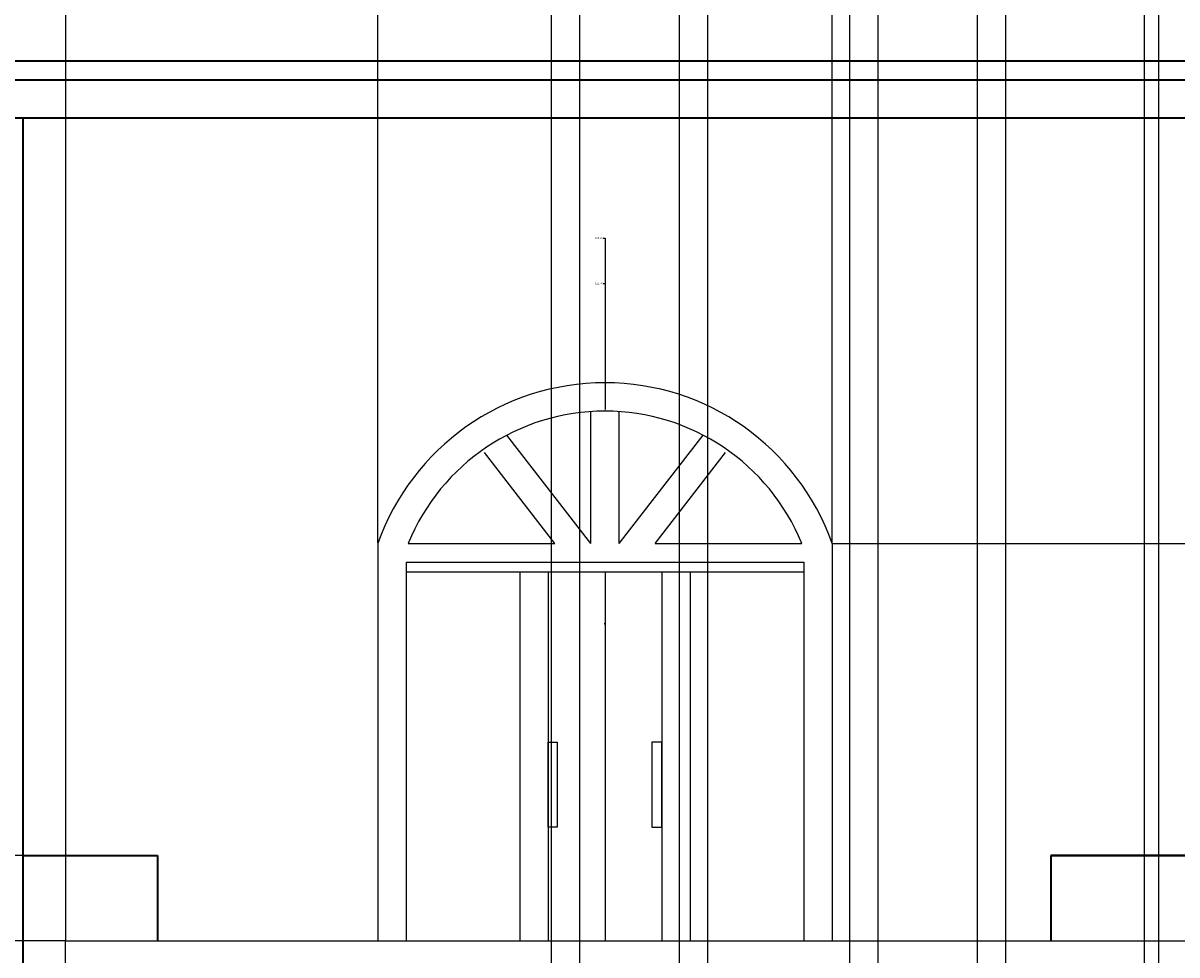
# Model space of a CAD drawing. Units: inches. Extents: x 2612 to 2948, y 481 to 865.
# Tile 3 of 7: x 2708 to 2830, y 561 to 659. Entities that reach past the tile are written whole.
import ezdxf

# ---------------------------------------------------------------- set-up
doc = ezdxf.new("R2010")
doc.units = ezdxf.units.IN
for name, color, linetype, lineweight in [('A-ANNO-DIMS', 2, 'Continuous', 18), ('A-DOOR', 4, 'Continuous', 25), ('A-ELEV', 7, 'Continuous', 35)]:
    doc.layers.add(name, color=color, linetype=linetype, lineweight=lineweight)
doc.styles.get("Standard").update_dxf_attribs({"font": 'arial.ttf'})
doc.dimstyles.get("Standard").update_dxf_attribs({"dimtxt": 0.18, "dimasz": 0.18, "dimexe": 0.18, "dimexo": 0.0625, "dimgap": 0.09, "dimtad": 0, "dimtih": 1, "dimtoh": 1, "dimdec": 4, "dimzin": 0, "dimdsep": 46, "dimtxsty": 'Standard', "dimcen": 0.09, "dimadec": 0, "dimazin": 0, "dimtfac": 1, "dimtdec": 4, "dimtofl": 0, "dimtmove": 0, "dimatfit": 3, "dimfxl": 1, "dimtolj": 1, "dimtzin": 0, "dimarcsym": 0})

# ---------------------------------------------------------------- blocks, each defined once
blk = doc.blocks.new('*D22')
at = {"layer": 'A-ANNO-DIMS', "color": 0, "lineweight": -2, "transparency": 16777216}
for p, q in [((2708.31, 648.98), (2708.31, 481.26)), ((2831.31, 570.98), (2831.31, 481.26)), ((2708.49, 481.44), (2769.53, 481.44)), ((2831.13, 481.44), (2770.09, 481.44))]:
    blk.add_line(p, q, dxfattribs=at)
at = {"layer": 'A-ANNO-DIMS', "color": 0, "transparency": 16777216}
for points in [[(2708.49, 481.47), (2708.49, 481.41), (2708.31, 481.44)], [(2831.13, 481.47), (2831.13, 481.41), (2831.31, 481.44)]]:
    blk.add_solid(points, dxfattribs=at)
at = {"layer": 'Defpoints', "color": 0, "transparency": 16777216}
for p in [(2708.31, 649.04), (2831.31, 571.04), (2831.31, 481.44)]:
    blk.add_point(p, dxfattribs=at)
at = {"layer": 'A-ANNO-DIMS', "color": 0, "transparency": 16777216, "insert": (2769.81, 481.44), "char_height": 0.18, "attachment_point": 5}
blk.add_mtext('\\A1;123', dxfattribs=at)
blk = doc.blocks.new('*D49')
at = {"layer": 'A-ANNO-DIMS', "color": 0, "lineweight": -2, "transparency": 16777216}
for p, q in [((2712.81, 562.11), (2712.81, 864.82)), ((2712.99, 864.64), (2729.09, 864.64)), ((2745.63, 864.64), (2729.53, 864.64)), ((2745.81, 604.11), (2745.81, 864.82))]:
    blk.add_line(p, q, dxfattribs=at)
at = {"layer": 'A-ANNO-DIMS', "color": 0, "transparency": 16777216}
for points in [[(2712.99, 864.67), (2712.99, 864.61), (2712.81, 864.64)], [(2745.63, 864.67), (2745.63, 864.61), (2745.81, 864.64)]]:
    blk.add_solid(points, dxfattribs=at)
at = {"layer": 'Defpoints', "color": 0, "transparency": 16777216}
for p in [(2745.81, 864.64), (2745.81, 604.04), (2712.81, 562.04)]:
    blk.add_point(p, dxfattribs=at)
at = {"layer": 'A-ANNO-DIMS', "color": 0, "transparency": 16777216, "insert": (2729.31, 864.64), "char_height": 0.18, "attachment_point": 5}
blk.add_mtext('\\A1;33', dxfattribs=at)
blk = doc.blocks.new('*D50')
at = {"layer": 'A-ANNO-DIMS', "color": 0, "lineweight": -2, "transparency": 16777216}
for p, q in [((2745.81, 604.11), (2745.81, 864.82)), ((2745.99, 864.64), (2769.58, 864.64)), ((2793.63, 864.64), (2770.03, 864.64)), ((2793.81, 604.11), (2793.81, 864.82))]:
    blk.add_line(p, q, dxfattribs=at)
at = {"layer": 'A-ANNO-DIMS', "color": 0, "transparency": 16777216}
for points in [[(2745.99, 864.67), (2745.99, 864.61), (2745.81, 864.64)], [(2793.63, 864.67), (2793.63, 864.61), (2793.81, 864.64)]]:
    blk.add_solid(points, dxfattribs=at)
at = {"layer": 'Defpoints', "color": 0, "transparency": 16777216}
for p in [(2793.81, 864.64), (2745.81, 604.04), (2793.81, 604.04)]:
    blk.add_point(p, dxfattribs=at)
at = {"layer": 'A-ANNO-DIMS', "color": 0, "transparency": 16777216, "insert": (2769.81, 864.64), "char_height": 0.18, "attachment_point": 5}
blk.add_mtext('\\A1;48', dxfattribs=at)
blk = doc.blocks.new('*D51')
at = {"layer": 'A-ANNO-DIMS', "color": 0, "lineweight": -2, "transparency": 16777216}
for p, q in [((2793.81, 604.11), (2793.81, 864.82)), ((2793.99, 864.64), (2810.09, 864.64)), ((2826.63, 864.64), (2810.53, 864.64)), ((2826.81, 562.11), (2826.81, 864.82))]:
    blk.add_line(p, q, dxfattribs=at)
at = {"layer": 'A-ANNO-DIMS', "color": 0, "transparency": 16777216}
for points in [[(2793.99, 864.67), (2793.99, 864.61), (2793.81, 864.64)], [(2826.63, 864.67), (2826.63, 864.61), (2826.81, 864.64)]]:
    blk.add_solid(points, dxfattribs=at)
at = {"layer": 'Defpoints', "color": 0, "transparency": 16777216}
for p in [(2826.81, 864.64), (2793.81, 604.04), (2826.81, 562.04)]:
    blk.add_point(p, dxfattribs=at)
at = {"layer": 'A-ANNO-DIMS', "color": 0, "transparency": 16777216, "insert": (2810.31, 864.64), "char_height": 0.18, "attachment_point": 5}
blk.add_mtext('\\A1;33', dxfattribs=at)
blk = doc.blocks.new('*D62')
at = {"layer": 'A-ANNO-DIMS', "color": 0, "lineweight": -2, "transparency": 16777216}
for p, q in [((2712.74, 562.04), (2612.53, 562.04)), ((2612.71, 561.86), (2612.71, 560.73)), ((2612.71, 559.22), (2612.71, 560.36)), ((2715.74, 559.04), (2612.53, 559.04))]:
    blk.add_line(p, q, dxfattribs=at)
at = {"layer": 'A-ANNO-DIMS', "color": 0, "transparency": 16777216}
for points in [[(2612.68, 561.86), (2612.74, 561.86), (2612.71, 562.04)], [(2612.68, 559.22), (2612.74, 559.22), (2612.71, 559.04)]]:
    blk.add_solid(points, dxfattribs=at)
at = {"layer": 'Defpoints', "color": 0, "transparency": 16777216}
for p in [(2612.71, 562.04), (2712.81, 562.04), (2715.81, 559.04)]:
    blk.add_point(p, dxfattribs=at)
at = {"layer": 'A-ANNO-DIMS', "color": 0, "transparency": 16777216, "insert": (2612.71, 560.54), "char_height": 0.18, "attachment_point": 5}
blk.add_mtext('\\A1;3', dxfattribs=at)
blk = doc.blocks.new('*D63')
at = {"layer": 'A-ANNO-DIMS', "color": 0, "lineweight": -2, "transparency": 16777216}
for p, q in [((2722.45, 571.04), (2612.53, 571.04)), ((2612.71, 570.86), (2612.71, 566.73)), ((2612.71, 562.22), (2612.71, 566.36)), ((2712.74, 562.04), (2612.53, 562.04))]:
    blk.add_line(p, q, dxfattribs=at)
at = {"layer": 'A-ANNO-DIMS', "color": 0, "transparency": 16777216}
for points in [[(2612.68, 570.86), (2612.74, 570.86), (2612.71, 571.04)], [(2612.68, 562.22), (2612.74, 562.22), (2612.71, 562.04)]]:
    blk.add_solid(points, dxfattribs=at)
at = {"layer": 'Defpoints', "color": 0, "transparency": 16777216}
for p in [(2612.71, 571.04), (2722.51, 571.04), (2712.81, 562.04)]:
    blk.add_point(p, dxfattribs=at)
at = {"layer": 'A-ANNO-DIMS', "color": 0, "transparency": 16777216, "insert": (2612.71, 566.54), "char_height": 0.18, "attachment_point": 5}
blk.add_mtext('\\A1;9', dxfattribs=at)
blk = doc.blocks.new('*D64')
at = {"layer": 'A-ANNO-DIMS', "color": 0, "lineweight": -2, "transparency": 16777216}
for p, q in [((2826.87, 562.04), (2948.09, 562.04)), ((2947.91, 561.86), (2947.91, 530.73)), ((2947.91, 499.22), (2947.91, 530.36)), ((2826.87, 499.04), (2948.09, 499.04))]:
    blk.add_line(p, q, dxfattribs=at)
at = {"layer": 'A-ANNO-DIMS', "color": 0, "transparency": 16777216}
for points in [[(2947.88, 561.86), (2947.94, 561.86), (2947.91, 562.04)], [(2947.88, 499.22), (2947.94, 499.22), (2947.91, 499.04)]]:
    blk.add_solid(points, dxfattribs=at)
at = {"layer": 'Defpoints', "color": 0, "transparency": 16777216}
for p in [(2826.81, 562.04), (2947.91, 562.04), (2826.81, 499.04)]:
    blk.add_point(p, dxfattribs=at)
at = {"layer": 'A-ANNO-DIMS', "color": 0, "transparency": 16777216, "insert": (2947.91, 530.54), "char_height": 0.18, "attachment_point": 5}
blk.add_mtext('\\A1;63', dxfattribs=at)
blk = doc.blocks.new('*D65')
at = {"layer": 'A-ANNO-DIMS', "color": 0, "lineweight": -2, "transparency": 16777216}
for p, q in [((2793.87, 604.04), (2948.09, 604.04)), ((2947.91, 603.86), (2947.91, 583.22)), ((2947.91, 562.22), (2947.91, 582.86)), ((2793.87, 562.04), (2948.09, 562.04))]:
    blk.add_line(p, q, dxfattribs=at)
at = {"layer": 'A-ANNO-DIMS', "color": 0, "transparency": 16777216}
for points in [[(2947.88, 603.86), (2947.94, 603.86), (2947.91, 604.04)], [(2947.88, 562.22), (2947.94, 562.22), (2947.91, 562.04)]]:
    blk.add_solid(points, dxfattribs=at)
at = {"layer": 'Defpoints', "color": 0, "transparency": 16777216}
for p in [(2793.81, 604.04), (2947.91, 604.04), (2793.81, 562.04)]:
    blk.add_point(p, dxfattribs=at)
at = {"layer": 'A-ANNO-DIMS', "color": 0, "transparency": 16777216, "insert": (2947.91, 583.04), "char_height": 0.18, "attachment_point": 5}
blk.add_mtext('\\A1;42', dxfattribs=at)
blk = doc.blocks.new('*D66')
at = {"layer": 'A-ANNO-DIMS', "color": 0, "lineweight": -2, "transparency": 16777216}
for p, q in [((2767.13, 711.98), (2767.13, 481.26)), ((2764.13, 708.98), (2764.13, 481.26)), ((2764.31, 481.44), (2765.48, 481.44)), ((2766.95, 481.44), (2765.78, 481.44))]:
    blk.add_line(p, q, dxfattribs=at)
at = {"layer": 'A-ANNO-DIMS', "color": 0, "transparency": 16777216}
for points in [[(2764.31, 481.47), (2764.31, 481.41), (2764.13, 481.44)], [(2766.95, 481.47), (2766.95, 481.41), (2767.13, 481.44)]]:
    blk.add_solid(points, dxfattribs=at)
at = {"layer": 'Defpoints', "color": 0, "transparency": 16777216}
for p in [(2767.13, 712.04), (2764.13, 709.04), (2767.13, 481.44)]:
    blk.add_point(p, dxfattribs=at)
at = {"layer": 'A-ANNO-DIMS', "color": 0, "transparency": 16777216, "insert": (2765.63, 481.44), "char_height": 0.18, "attachment_point": 5}
blk.add_mtext('\\A1;3', dxfattribs=at)
blk = doc.blocks.new('*D67')
at = {"layer": 'A-ANNO-DIMS', "color": 0, "lineweight": -2, "transparency": 16777216}
for p, q in [((2767.13, 711.98), (2767.13, 481.26)), ((2777.63, 711.98), (2777.63, 481.26)), ((2767.31, 481.44), (2772.06, 481.44)), ((2777.45, 481.44), (2772.7, 481.44))]:
    blk.add_line(p, q, dxfattribs=at)
at = {"layer": 'A-ANNO-DIMS', "color": 0, "transparency": 16777216}
for points in [[(2767.31, 481.47), (2767.31, 481.41), (2767.13, 481.44)], [(2777.45, 481.47), (2777.45, 481.41), (2777.63, 481.44)]]:
    blk.add_solid(points, dxfattribs=at)
at = {"layer": 'Defpoints', "color": 0, "transparency": 16777216}
for p in [(2767.13, 712.04), (2777.63, 712.04), (2777.63, 481.44)]:
    blk.add_point(p, dxfattribs=at)
at = {"layer": 'A-ANNO-DIMS', "color": 0, "transparency": 16777216, "insert": (2772.38, 481.44), "char_height": 0.18, "attachment_point": 5}
blk.add_mtext('\\A1;10.5', dxfattribs=at)
blk = doc.blocks.new('*D68')
at = {"layer": 'A-ANNO-DIMS', "color": 0, "lineweight": -2, "transparency": 16777216}
for p, q in [((2777.63, 711.98), (2777.63, 481.26)), ((2780.63, 711.98), (2780.63, 481.26)), ((2777.81, 481.44), (2778.98, 481.44)), ((2780.45, 481.44), (2779.28, 481.44))]:
    blk.add_line(p, q, dxfattribs=at)
at = {"layer": 'A-ANNO-DIMS', "color": 0, "transparency": 16777216}
for points in [[(2777.81, 481.47), (2777.81, 481.41), (2777.63, 481.44)], [(2780.45, 481.47), (2780.45, 481.41), (2780.63, 481.44)]]:
    blk.add_solid(points, dxfattribs=at)
at = {"layer": 'Defpoints', "color": 0, "transparency": 16777216}
for p in [(2777.63, 712.04), (2780.63, 712.04), (2780.63, 481.44)]:
    blk.add_point(p, dxfattribs=at)
at = {"layer": 'A-ANNO-DIMS', "color": 0, "transparency": 16777216, "insert": (2779.13, 481.44), "char_height": 0.18, "attachment_point": 5}
blk.add_mtext('\\A1;3', dxfattribs=at)
blk = doc.blocks.new('*D69')
at = {"layer": 'A-ANNO-DIMS', "color": 0, "lineweight": -2, "transparency": 16777216}
for p, q in [((2780.63, 711.98), (2780.63, 481.26)), ((2795.63, 711.98), (2795.63, 481.26)), ((2780.81, 481.44), (2787.92, 481.44)), ((2795.45, 481.44), (2788.34, 481.44))]:
    blk.add_line(p, q, dxfattribs=at)
at = {"layer": 'A-ANNO-DIMS', "color": 0, "transparency": 16777216}
for points in [[(2780.81, 481.47), (2780.81, 481.41), (2780.63, 481.44)], [(2795.45, 481.47), (2795.45, 481.41), (2795.63, 481.44)]]:
    blk.add_solid(points, dxfattribs=at)
at = {"layer": 'Defpoints', "color": 0, "transparency": 16777216}
for p in [(2780.63, 712.04), (2795.63, 712.04), (2795.63, 481.44)]:
    blk.add_point(p, dxfattribs=at)
at = {"layer": 'A-ANNO-DIMS', "color": 0, "transparency": 16777216, "insert": (2788.13, 481.44), "char_height": 0.18, "attachment_point": 5}
blk.add_mtext('\\A1;15', dxfattribs=at)
blk = doc.blocks.new('*D70')
at = {"layer": 'A-ANNO-DIMS', "color": 0, "lineweight": -2, "transparency": 16777216}
for p, q in [((2795.63, 711.98), (2795.63, 481.26)), ((2798.63, 711.98), (2798.63, 481.26)), ((2795.81, 481.44), (2796.98, 481.44)), ((2798.45, 481.44), (2797.28, 481.44))]:
    blk.add_line(p, q, dxfattribs=at)
at = {"layer": 'A-ANNO-DIMS', "color": 0, "transparency": 16777216}
for points in [[(2795.81, 481.47), (2795.81, 481.41), (2795.63, 481.44)], [(2798.45, 481.47), (2798.45, 481.41), (2798.63, 481.44)]]:
    blk.add_solid(points, dxfattribs=at)
at = {"layer": 'Defpoints', "color": 0, "transparency": 16777216}
for p in [(2795.63, 712.04), (2798.63, 712.04), (2798.63, 481.44)]:
    blk.add_point(p, dxfattribs=at)
at = {"layer": 'A-ANNO-DIMS', "color": 0, "transparency": 16777216, "insert": (2797.13, 481.44), "char_height": 0.18, "attachment_point": 5}
blk.add_mtext('\\A1;3', dxfattribs=at)
blk = doc.blocks.new('*D71')
at = {"layer": 'A-ANNO-DIMS', "color": 0, "lineweight": -2, "transparency": 16777216}
for p, q in [((2798.63, 711.98), (2798.63, 481.26)), ((2809.13, 711.98), (2809.13, 481.26)), ((2798.81, 481.44), (2803.56, 481.44)), ((2808.95, 481.44), (2804.2, 481.44))]:
    blk.add_line(p, q, dxfattribs=at)
at = {"layer": 'A-ANNO-DIMS', "color": 0, "transparency": 16777216}
for points in [[(2798.81, 481.47), (2798.81, 481.41), (2798.63, 481.44)], [(2808.95, 481.47), (2808.95, 481.41), (2809.13, 481.44)]]:
    blk.add_solid(points, dxfattribs=at)
at = {"layer": 'Defpoints', "color": 0, "transparency": 16777216}
for p in [(2798.63, 712.04), (2809.13, 712.04), (2809.13, 481.44)]:
    blk.add_point(p, dxfattribs=at)
at = {"layer": 'A-ANNO-DIMS', "color": 0, "transparency": 16777216, "insert": (2803.88, 481.44), "char_height": 0.18, "attachment_point": 5}
blk.add_mtext('\\A1;10.5', dxfattribs=at)
blk = doc.blocks.new('*D72')
at = {"layer": 'A-ANNO-DIMS', "color": 0, "lineweight": -2, "transparency": 16777216}
for p, q in [((2809.13, 711.98), (2809.13, 481.26)), ((2812.13, 708.98), (2812.13, 481.26)), ((2809.31, 481.44), (2810.48, 481.44)), ((2811.95, 481.44), (2810.78, 481.44))]:
    blk.add_line(p, q, dxfattribs=at)
at = {"layer": 'A-ANNO-DIMS', "color": 0, "transparency": 16777216}
for points in [[(2809.31, 481.47), (2809.31, 481.41), (2809.13, 481.44)], [(2811.95, 481.47), (2811.95, 481.41), (2812.13, 481.44)]]:
    blk.add_solid(points, dxfattribs=at)
at = {"layer": 'Defpoints', "color": 0, "transparency": 16777216}
for p in [(2809.13, 712.04), (2812.13, 709.04), (2812.13, 481.44)]:
    blk.add_point(p, dxfattribs=at)
at = {"layer": 'A-ANNO-DIMS', "color": 0, "transparency": 16777216, "insert": (2810.63, 481.44), "char_height": 0.18, "attachment_point": 5}
blk.add_mtext('\\A1;3', dxfattribs=at)
blk = doc.blocks.new('*D73')
at = {"layer": 'A-ANNO-DIMS', "color": 0, "lineweight": -2, "transparency": 16777216}
for p, q in [((2812.13, 708.98), (2812.13, 481.26)), ((2828.31, 708.98), (2828.31, 481.26)), ((2812.31, 481.44), (2819.76, 481.44)), ((2828.13, 481.44), (2820.67, 481.44))]:
    blk.add_line(p, q, dxfattribs=at)
at = {"layer": 'A-ANNO-DIMS', "color": 0, "transparency": 16777216}
for points in [[(2812.31, 481.47), (2812.31, 481.41), (2812.13, 481.44)], [(2828.13, 481.47), (2828.13, 481.41), (2828.31, 481.44)]]:
    blk.add_solid(points, dxfattribs=at)
at = {"layer": 'Defpoints', "color": 0, "transparency": 16777216}
for p in [(2812.13, 709.04), (2828.31, 709.04), (2828.31, 481.44)]:
    blk.add_point(p, dxfattribs=at)
at = {"layer": 'A-ANNO-DIMS', "color": 0, "transparency": 16777216, "insert": (2820.22, 481.44), "char_height": 0.18, "attachment_point": 5}
blk.add_mtext('\\A1;16.177', dxfattribs=at)
blk = doc.blocks.new('*D74')
at = {"layer": 'A-ANNO-DIMS', "color": 0, "lineweight": -2, "transparency": 16777216}
for p, q in [((2831.31, 711.98), (2831.31, 481.26)), ((2828.31, 708.98), (2828.31, 481.26)), ((2828.49, 481.44), (2829.66, 481.44)), ((2831.13, 481.44), (2829.96, 481.44))]:
    blk.add_line(p, q, dxfattribs=at)
at = {"layer": 'A-ANNO-DIMS', "color": 0, "transparency": 16777216}
for points in [[(2828.49, 481.47), (2828.49, 481.41), (2828.31, 481.44)], [(2831.13, 481.47), (2831.13, 481.41), (2831.31, 481.44)]]:
    blk.add_solid(points, dxfattribs=at)
at = {"layer": 'Defpoints', "color": 0, "transparency": 16777216}
for p in [(2831.31, 712.04), (2828.31, 709.04), (2831.31, 481.44)]:
    blk.add_point(p, dxfattribs=at)
at = {"layer": 'A-ANNO-DIMS', "color": 0, "transparency": 16777216, "insert": (2829.81, 481.44), "char_height": 0.18, "attachment_point": 5}
blk.add_mtext('\\A1;3', dxfattribs=at)
blk = doc.blocks.new('*D93')
at = {"layer": 'A-ANNO-DIMS', "color": 0, "lineweight": -2, "transparency": 16777216}
for p, q in [((2769.63, 636.3), (2769.81, 636.3)), ((2769.81, 636.3), (2769.81, 621.21)), ((2769.72, 595.57), (2769.9, 595.57)), ((2769.81, 595.48), (2769.81, 595.66))]:
    blk.add_line(p, q, dxfattribs=at)
at = {"layer": 'A-ANNO-DIMS', "color": 0, "transparency": 16777216}
blk.add_solid([(2769.84, 621.21), (2769.78, 621.21), (2769.81, 621.03)], dxfattribs=at)
at = {"layer": 'Defpoints', "color": 0, "transparency": 16777216}
for p in [(2769.81, 621.03), (2769.81, 595.57)]:
    blk.add_point(p, dxfattribs=at)
at = {"layer": 'A-ANNO-DIMS', "color": 0, "transparency": 16777216, "insert": (2769.15, 636.3), "char_height": 0.18, "attachment_point": 5}
blk.add_mtext('\\A1;R25.45', dxfattribs=at)
blk = doc.blocks.new('*D94')
at = {"layer": 'A-ANNO-DIMS', "color": 0, "lineweight": -2, "transparency": 16777216}
for p, q in [((2769.63, 631.5), (2769.81, 631.5)), ((2769.81, 631.5), (2769.81, 618.21)), ((2769.72, 595.57), (2769.9, 595.57)), ((2769.81, 595.48), (2769.81, 595.66))]:
    blk.add_line(p, q, dxfattribs=at)
at = {"layer": 'A-ANNO-DIMS', "color": 0, "transparency": 16777216}
blk.add_solid([(2769.84, 618.21), (2769.78, 618.21), (2769.81, 618.03)], dxfattribs=at)
at = {"layer": 'Defpoints', "color": 0, "transparency": 16777216}
for p in [(2769.81, 618.03), (2769.81, 595.57)]:
    blk.add_point(p, dxfattribs=at)
at = {"layer": 'A-ANNO-DIMS', "color": 0, "transparency": 16777216, "insert": (2769.15, 631.5), "char_height": 0.18, "attachment_point": 5}
blk.add_mtext('\\A1;R22.45', dxfattribs=at)

msp = doc.modelspace()

# ---------------------------------------------------------------- linework, layer by layer
at = {"layer": 'A-DOOR'}
for p, q in [((2768.3074, 604.0443), (2768.3074, 618.0252)), ((2771.3074, 604.0443), (2771.3074, 618.0252)), ((2768.3074, 604.0443), (2759.4335, 615.4847)), ((2771.3074, 604.0443), (2780.1813, 615.4847)), ((2764.5107, 604.0443), (2757.0631, 613.646)), ((2775.1041, 604.0443), (2782.5518, 613.646)), ((2745.8074, 604.0443), (2745.8074, 562.0443)), ((2749.0157, 604.0443), (2764.5107, 604.0443)), ((2775.1041, 604.0443), (2790.5991, 604.0443)), ((2793.8074, 604.0443), (2793.8074, 562.0443)), ((2748.8074, 602.0443), (2748.8074, 562.0443)), ((2748.8074, 602.0443), (2790.8074, 602.0443)), ((2790.8074, 602.0443), (2790.8074, 562.0443)), ((2748.8074, 601.0443), (2790.8074, 601.0443)), ((2760.8074, 601.0443), (2760.8074, 562.0443)), ((2763.8074, 601.0443), (2763.8074, 562.0443)), ((2769.8074, 601.0443), (2769.8074, 562.0443)), ((2775.8074, 601.0443), (2775.8074, 562.0443)), ((2778.8074, 601.0443), (2778.8074, 562.0443)), ((2712.8074, 529.0443), (2712.8074, 562.0443)), ((2712.8074, 562.0443), (2826.8074, 562.0443)), ((2712.8074, 499.0443), (2712.8074, 562.0443)), ((2745.8074, 562.0443), (2793.8074, 562.0443)), ((2826.8074, 499.0443), (2826.8074, 562.0443))]:
    msp.add_line(p, q, dxfattribs=at)
for points in [[(2763.8074, 583.0443), (2764.7611, 583.0443), (2764.7611, 574.0443), (2763.8074, 574.0443)], [(2775.8074, 583.0443), (2774.7732, 583.0443), (2774.7732, 574.0443), (2775.8074, 574.0443)]]:
    msp.add_lwpolyline(points, close=True, dxfattribs=at)
for radius, start, end in [(25.4507, 19.438284, 160.561716), (22.4507, 22.164123, 157.835877)]:
    msp.add_arc((2769.8074, 595.5745), radius, start, end, dxfattribs=at)
at = {"layer": 'A-ELEV'}
for p, q in [((2642.3074, 655.0443), (2918.3074, 655.0443)), ((2642.3074, 653.0443), (2918.3074, 653.0443)), ((2642.3074, 649.0443), (2918.3074, 649.0443)), ((2708.3074, 499.0443), (2708.3074, 649.0443)), ((2717.3074, 649.0443), (2822.3074, 649.0443)), ((2708.3074, 571.0443), (2722.5147, 571.0443)), ((2708.3074, 571.0443), (2722.5147, 571.0443)), ((2722.5147, 571.0443), (2722.5147, 562.0443)), ((2816.9214, 571.0443), (2900.3074, 571.0443)), ((2831.3074, 571.0443), (2816.9214, 571.0443)), ((2816.9214, 571.0443), (2816.9214, 562.0443))]:
    msp.add_line(p, q, dxfattribs=at)

# ---------------------------------------------------------------- dimensions: what is measured, and where the dimension line sits
at = {"layer": 'A-ANNO-DIMS'}
for base, p1, p2, override, picture, middle in [((2745.8074, 864.6443), (2712.8074, 562.0443), (2745.8074, 604.0443), {"dimdec": 0, "dimlfac": 1, "dimrnd": 0, "dimzin": 0, "dimdsep": 46, "dimlunit": 2}, '*D49', (2729.3074, 864.6443)), ((2793.8074, 864.6443), (2745.8074, 604.0443), (2793.8074, 604.0443), {"dimdec": 0, "dimlfac": 1, "dimrnd": 0, "dimzin": 0, "dimdsep": 46, "dimlunit": 2}, '*D50', (2769.8074, 864.6443)), ((2826.8074, 864.6443), (2793.8074, 604.0443), (2826.8074, 562.0443), {"dimdec": 0, "dimlfac": 1, "dimrnd": 0, "dimzin": 0, "dimdsep": 46, "dimlunit": 2}, '*D51', (2810.3074, 864.6443)), ((2767.1304, 481.4443), (2764.1304, 709.0443), (2767.1304, 712.0443), {"dimdec": 0, "dimlfac": 1, "dimrnd": 0, "dimzin": 0, "dimdsep": 46, "dimlunit": 2}, '*D66', (2765.6304, 481.4443)), ((2777.6304, 481.4443), (2767.1304, 712.0443), (2777.6304, 712.0443), {"dimdec": 1, "dimlfac": 1, "dimrnd": 0, "dimzin": 0, "dimdsep": 46, "dimlunit": 2}, '*D67', (2772.3804, 481.4443)), ((2780.6304, 481.4443), (2777.6304, 712.0443), (2780.6304, 712.0443), {"dimdec": 0, "dimlfac": 1, "dimrnd": 0, "dimzin": 0, "dimdsep": 46, "dimlunit": 2}, '*D68', (2779.1304, 481.4443)), ((2795.6304, 481.4443), (2780.6304, 712.0443), (2795.6304, 712.0443), {"dimdec": 0, "dimlfac": 1, "dimrnd": 0, "dimzin": 0, "dimdsep": 46, "dimlunit": 2}, '*D69', (2788.1304, 481.4443)), ((2798.6304, 481.4443), (2795.6304, 712.0443), (2798.6304, 712.0443), {"dimdec": 0, "dimlfac": 1, "dimrnd": 0, "dimzin": 0, "dimdsep": 46, "dimlunit": 2}, '*D70', (2797.1304, 481.4443)), ((2809.1304, 481.4443), (2798.6304, 712.0443), (2809.1304, 712.0443), {"dimdec": 1, "dimlfac": 1, "dimrnd": 0, "dimzin": 0, "dimdsep": 46, "dimlunit": 2}, '*D71', (2803.8804, 481.4443)), ((2812.1304, 481.4443), (2809.1304, 712.0443), (2812.1304, 709.0443), {"dimdec": 0, "dimlfac": 1, "dimrnd": 0, "dimzin": 0, "dimdsep": 46, "dimlunit": 2}, '*D72', (2810.6304, 481.4443)), ((2831.3074, 481.4443), (2828.3074, 709.0443), (2831.3074, 712.0443), {"dimdec": 0, "dimlfac": 1, "dimrnd": 0, "dimzin": 0, "dimdsep": 46, "dimlunit": 2}, '*D74', (2829.8074, 481.4443)), ((2828.3074, 481.4443), (2812.1304, 709.0443), (2828.3074, 709.0443), {"dimdec": 3, "dimlfac": 1, "dimrnd": 0, "dimzin": 0, "dimdsep": 46, "dimlunit": 2}, '*D73', (2820.2189, 481.4443)), ((2831.3074, 481.4443), (2708.3074, 649.0443), (2831.3074, 571.0443), {"dimdec": 0, "dimlfac": 1, "dimrnd": 0, "dimzin": 0, "dimdsep": 46, "dimlunit": 2}, '*D22', (2769.8074, 481.4443))]:
    dim = msp.add_linear_dim(base=base, p1=p1, p2=p2, dimstyle='Standard', override=override, dxfattribs=at)
    dim.commit()
    dim.dimension.update_dxf_attribs({"geometry": picture, "text_midpoint": middle})
for mpoint, picture, middle in [((2769.807, 621.0252), '*D93', (2769.1462, 636.2956)), ((2769.807, 618.0252), '*D94', (2769.1462, 631.4956))]:
    dim = msp.add_radius_dim(center=(2769.8074, 595.5745), mpoint=mpoint, dimstyle='Standard', override={"dimdec": 2, "dimlfac": 1, "dimrnd": 0, "dimzin": 0, "dimdsep": 46, "dimlunit": 2}, dxfattribs=at)
    dim.commit()
    dim.dimension.update_dxf_attribs({"geometry": picture, "text_midpoint": middle, "dimtype": 164})
for base, p1, p2, picture, middle in [((2947.9074, 604.0443), (2793.8074, 562.0443), (2793.8074, 604.0443), '*D65', (2947.9074, 583.0443)), ((2612.7074, 571.0443), (2712.8074, 562.0443), (2722.5147, 571.0443), '*D63', (2612.7074, 566.5443)), ((2612.7074, 562.0443), (2715.8074, 559.0443), (2712.8074, 562.0443), '*D62', (2612.7074, 560.5443)), ((2947.9074, 562.0443), (2826.8074, 499.0443), (2826.8074, 562.0443), '*D64', (2947.9074, 530.5443))]:
    dim = msp.add_linear_dim(base=base, p1=p1, p2=p2, angle=90, dimstyle='Standard', override={"dimdec": 0, "dimlfac": 1, "dimrnd": 0, "dimzin": 0, "dimdsep": 46, "dimlunit": 2}, dxfattribs=at)
    dim.commit()
    dim.dimension.update_dxf_attribs({"geometry": picture, "text_midpoint": middle})

doc.saveas('drawing.dxf')
